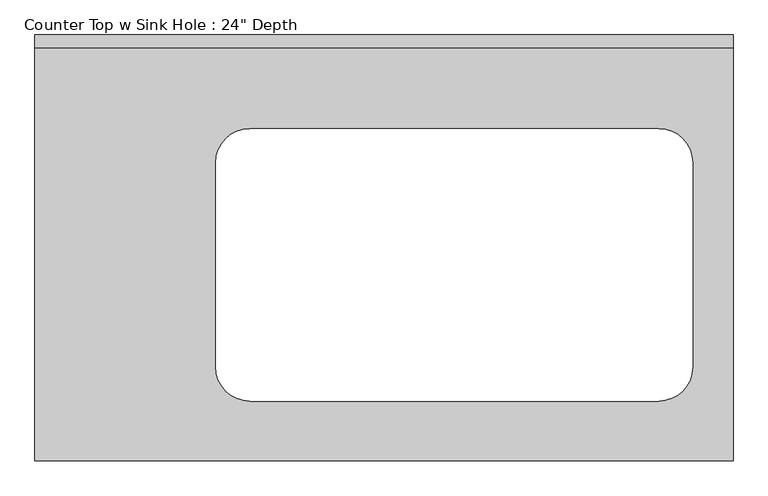
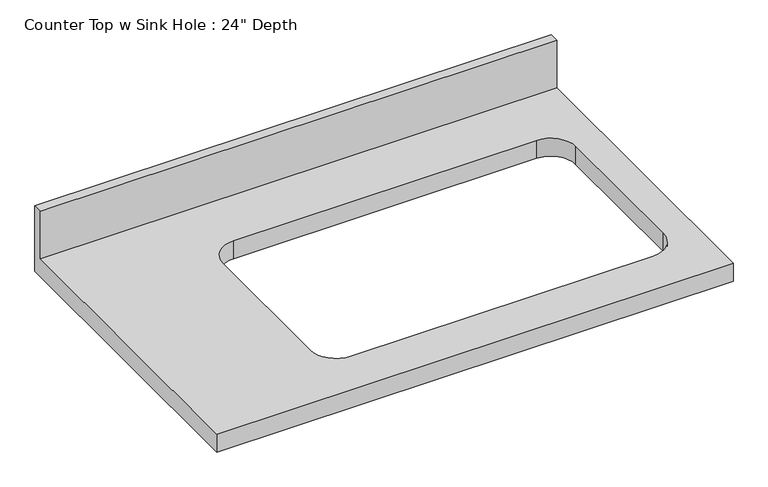
"""IFC4 building model written with IfcOpenShell, lengths in millimetres: furniture geometry."""

from ifc_helpers import new_model, si_unit, frame, origin, place, context, project, spatial, polyline, circle_curve, source, transform, mapped, element, save
from ifc_brep_helpers import plane_surface, revolved_surface, advanced_brep


def furniture_738e865d(model_context):
    return source(origin(), model_context, "Body", "AdvancedBrep", [
        advanced_brep(
        [(-1200.4622951, -635.0, 914.4), (-159.0622951, -635.0, 914.4), (-159.0622951, -19.05, 914.4), (-1200.4622951, -19.05, 914.4), (-879.7872951, -139.7, 914.4), (-270.1872951, -139.7, 914.4), (-219.3872951, -190.5, 914.4), (-219.3872951, -495.3, 914.4), (-270.1872951, -546.1, 914.4), (-879.7872951, -546.1, 914.4), (-930.5872951, -495.3, 914.4), (-930.5872951, -190.5, 914.4), (-159.0622951, 0.0, 876.3), (-159.0622951, -635.0, 876.3), (-1200.4622951, -635.0, 876.3), (-1200.4622951, 0.0, 876.3), (-270.1872951, -139.7, 876.3), (-879.7872951, -139.7, 876.3), (-930.5872951, -190.5, 876.3), (-930.5872951, -495.3, 876.3), (-879.7872951, -546.1, 876.3), (-270.1872951, -546.1, 876.3), (-219.3872951, -495.3, 876.3), (-219.3872951, -190.5, 876.3), (-1200.4622951, 0.0, 1016.0), (-159.0622951, 0.0, 1016.0), (-1200.4622951, -19.05, 1016.0), (-159.0622951, -19.05, 1016.0)],
        [
            (0, 1),
            (1, 2),
            (2, 3),
            (3, 0),
            (4, 5),
            (5, 6, circle_curve(frame((-270.1872951, -190.5, 914.4), z_axis=(0.0, 0.0, -1.0), x_axis=(1.0, 0.0, 0.0)), 50.8)),
            (6, 7),
            (7, 8, circle_curve(frame((-270.1872951, -495.3, 914.4), z_axis=(0.0, 0.0, -1.0), x_axis=(1.0, 0.0, 0.0)), 50.8)),
            (8, 9),
            (9, 10, circle_curve(frame((-879.7872951, -495.3, 914.4), z_axis=(0.0, 0.0, -1.0), x_axis=(1.0, 0.0, 0.0)), 50.8)),
            (10, 11),
            (11, 4, circle_curve(frame((-879.7872951, -190.5, 914.4), z_axis=(0.0, 0.0, -1.0), x_axis=(1.0, 0.0, 0.0)), 50.8)),
            (12, 13),
            (13, 14),
            (14, 15),
            (15, 12),
            (16, 17),
            (17, 18, circle_curve(frame((-879.7872951, -190.5, 876.3), z_axis=(0.0, 0.0, 1.0), x_axis=(1.0, 0.0, 0.0)), 50.8)),
            (18, 19),
            (19, 20, circle_curve(frame((-879.7872951, -495.3, 876.3), z_axis=(0.0, 0.0, 1.0), x_axis=(1.0, 0.0, 0.0)), 50.8)),
            (20, 21),
            (21, 22, circle_curve(frame((-270.1872951, -495.3, 876.3), z_axis=(0.0, 0.0, 1.0), x_axis=(1.0, 0.0, 0.0)), 50.8)),
            (22, 23),
            (23, 16, circle_curve(frame((-270.1872951, -190.5, 876.3), z_axis=(0.0, 0.0, 1.0), x_axis=(1.0, 0.0, 0.0)), 50.8)),
            (15, 24),
            (24, 25),
            (25, 12),
            (14, 0),
            (3, 26),
            (26, 24),
            (13, 1),
            (25, 27),
            (27, 2),
            (26, 27),
            (4, 17),
            (16, 5),
            (11, 18),
            (10, 19),
            (9, 20),
            (8, 21),
            (7, 22),
            (6, 23),
        ],
        [
            plane_surface(frame((-1200.4622951, 0.0, 914.4), z_axis=(0.0, 0.0, 1.0), x_axis=(-1.0, 0.0, 0.0))),
            plane_surface(frame((-1200.4622951, 0.0, 876.3), z_axis=(0.0, 0.0, -1.0), x_axis=(1.0, 0.0, 0.0))),
            plane_surface(frame((-159.0622951, 0.0, 914.4), z_axis=(0.0, 1.0, 0.0), x_axis=(0.0, 0.0, -1.0))),
            plane_surface(frame((-1200.4622951, 0.0, 914.4), z_axis=(-1.0, 0.0, 0.0), x_axis=(0.0, 0.0, -1.0))),
            plane_surface(frame((-1200.4622951, -635.0, 914.4), z_axis=(0.0, -1.0, 0.0), x_axis=(0.0, 0.0, -1.0))),
            plane_surface(frame((-159.0622951, -635.0, 914.4), z_axis=(1.0, 0.0, 0.0), x_axis=(0.0, 0.0, -1.0))),
            plane_surface(frame((-1200.4622951, 0.0, 1016.0), z_axis=(0.0, 0.0, 1.0), x_axis=(0.0, -1.0, 0.0))),
            plane_surface(frame((-1200.4622951, -19.05, 1016.0), z_axis=(0.0, -1.0, 0.0), x_axis=(0.0, 0.0, -1.0))),
            plane_surface(frame((-270.1872951, -139.7, 914.4), z_axis=(0.0, -1.0, 0.0), x_axis=(0.0, 0.0, -1.0))),
            revolved_surface(polyline([(-828.9872951000001, -190.5, 914.4), (-828.9872951000001, -190.5, 876.3)]), (-879.7872951, -190.5, 876.3), (0.0, 0.0, 1.0)),
            plane_surface(frame((-930.5872951, -190.5, 914.4), z_axis=(1.0, 0.0, 0.0), x_axis=(0.0, 0.0, -1.0))),
            revolved_surface(polyline([(-828.9872951000001, -495.3, 914.4), (-828.9872951000001, -495.3, 876.3)]), (-879.7872951, -495.3, 876.3), (0.0, 0.0, 1.0)),
            plane_surface(frame((-879.7872951, -546.1, 914.4), z_axis=(0.0, 1.0, 0.0), x_axis=(0.0, 0.0, -1.0))),
            revolved_surface(polyline([(-219.38729509999996, -495.3, 914.4), (-219.38729509999996, -495.3, 876.3)]), (-270.1872951, -495.3, 876.3), (0.0, 0.0, 1.0)),
            plane_surface(frame((-219.3872951, -495.3, 914.4), z_axis=(-1.0, 0.0, 0.0), x_axis=(0.0, 0.0, -1.0))),
            revolved_surface(polyline([(-219.38729509999996, -190.5, 914.4), (-219.38729509999996, -190.5, 876.3)]), (-270.1872951, -190.5, 876.3), (0.0, 0.0, 1.0)),
        ],
        [
            (0, [[1, 2, 3, 4], [5, 6, 7, 8, 9, 10, 11, 12]]),
            (1, [[13, 14, 15, 16], [17, 18, 19, 20, 21, 22, 23, 24]]),
            (2, [[-16, 25, 26, 27]]),
            (3, [[-15, 28, -4, 29, 30, -25]]),
            (4, [[-1, -28, -14, 31]]),
            (5, [[-13, -27, 32, 33, -2, -31]]),
            (6, [[-30, 34, -32, -26]]),
            (7, [[-34, -29, -3, -33]]),
            (8, [[35, -17, 36, -5]]),
            (9, [[-35, -12, 37, -18]]),
            (10, [[-37, -11, 38, -19]]),
            (11, [[-38, -10, 39, -20]]),
            (12, [[-39, -9, 40, -21]]),
            (13, [[-40, -8, 41, -22]]),
            (14, [[-41, -7, 42, -23]]),
            (15, [[-36, -24, -42, -6]]),
        ],
    ),
    ])


if __name__ == "__main__":
    model = new_model("IFC4")
    model_context = context("Model", 3, world=origin())
    ifc_project = project(units=[si_unit("LENGTHUNIT", "METRE", prefix="MILLI")], contexts=[model_context])
    site = spatial("IfcSite", under=ifc_project)
    building = spatial("IfcBuilding", under=site)
    placement = place(None, origin())
    furniture_shape = furniture_738e865d(model_context)
    element("IfcFurniture", 1, ObjectType="Counter Top w Sink Hole : 24\" Depth", at=placement, inside=building, context=model_context, shape_type="MappedRepresentation", body=[
        mapped(furniture_shape, transform((0.0, 0.0, 0.0), x_axis=(1.0, 0.0, 0.0), y_axis=(0.0, 1.0, 0.0), z_axis=(0.0, 0.0, 1.0))),
    ])
    save(model, "model.ifc")

# Revit data of these elements
# Type "Counter Top w Sink Hole : 24\" Depth"
#   Assembly Code = "C1030400"
#   Counter Thickness = 0' - 1 1/2"
#   Depth = 2' - 1"
#   Height = 3' - 0"
#   Length [instance default] = 8' - 0"
#   Sink Location [instance default] = 2' - 0"
#   Sink Location To Wall [instance default] = 0' - 6"
#   Sink Opening Depth [instance default] = 1' - 3"
#   Sink Opening Width [instance default] = 2' - 3"
#   Counter Top Material = none
#   Default Elevation = 0
# Element 1 (IfcFurniture, "Counter Top w Sink Hole : 24\" Depth")
#   Length = 3' - 5"
#   Sink Location = 2' - 0 5/8"
#   Materials on its faces: "Counter Top"
# Materials
#   "Counter Top": class "Wood", colour RGB 226 177 128, transparency 0
